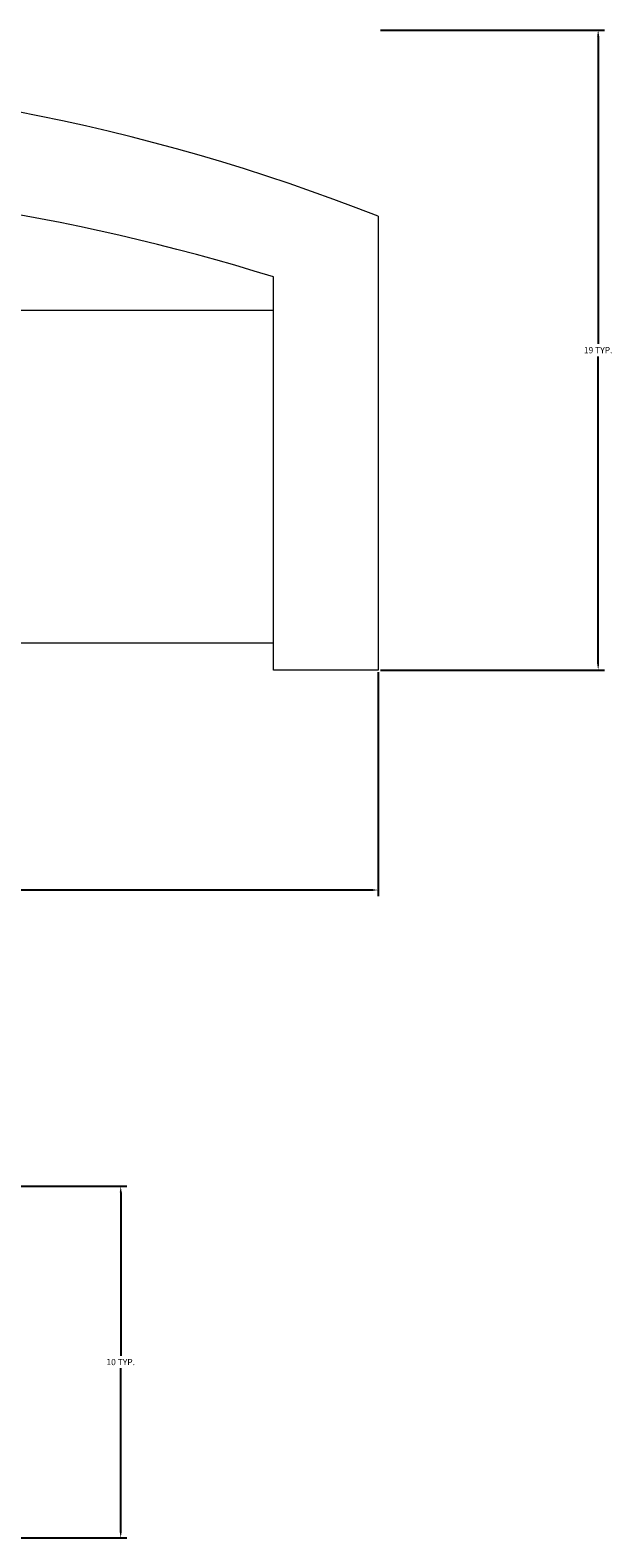
# Model space of a CAD drawing. Units: feet. Extents: x 2219 to 3039, y 1768 to 2369.
# Tile 10 of 16: x 2764 to 2781, y 2273 to 2317. Entities that reach past the tile are written whole.
import ezdxf

# ---------------------------------------------------------------- set-up
doc = ezdxf.new("R2010")
doc.units = ezdxf.units.FT
doc.layers.add('A-ANNO-DIMS', color=2, linetype='Continuous', lineweight=18)
doc.layers.add('A-FURN', color=8, linetype='Continuous', lineweight=18)
doc.styles.get("Standard").update_dxf_attribs({"font": 'arial.ttf'})
doc.dimstyles.get("Standard").update_dxf_attribs({"dimtxt": 0.18, "dimasz": 0.18, "dimexe": 0.18, "dimexo": 0.0625, "dimgap": 0.09, "dimtad": 0, "dimtih": 1, "dimtoh": 1, "dimdec": 4, "dimzin": 0, "dimdsep": 46, "dimtxsty": 'Standard', "dimcen": 0.09, "dimadec": 0, "dimazin": 0, "dimtfac": 1, "dimtdec": 4, "dimtofl": 0, "dimtmove": 0, "dimatfit": 3, "dimfxl": 1, "dimtolj": 1, "dimtzin": 0, "dimarcsym": 0})

# ---------------------------------------------------------------- blocks, each defined once
blk = doc.blocks.new('Sofa - Roundback 7 ft.')
for p, q in [((-12.00002, -32.4421), (-12.00003, -6.5971)), ((11.99997, -32.4421), (11.99998, -6.5971)), ((-36.000027, -34), (-36.000027, -11.4696)), ((35.99998, -34), (35.99998, -11.4696)), ((-35.999844, -13.3819), (35.9998, -13.3819)), ((-36.000027, -32.4421), (35.99998, -32.4421))]:
    blk.add_line(p, q)
for points in [[(-36.000027, -34), (-42.000027, -34), (-42.000027, -8)], [(41.99998, -8), (41.99998, -34), (35.99998, -34)]]:
    blk.add_lwpolyline(points)
for centre, radius, start, end in [((0, -114.25), 114.25, 68.43141, 111.5686), ((-0.00001, -127.1968), 121.1968, 72.72033, 107.2797)]:
    blk.add_arc(centre, radius, start, end)
blk = doc.blocks.new('*D24')
at = {"layer": 'A-ANNO-DIMS', "color": 0, "lineweight": -2, "transparency": 16777216}
for p, q in [((2731.366, 2298.238), (2731.366, 2291.74)), ((2773.903, 2298.238), (2773.903, 2291.74)), ((2731.546, 2291.92), (2751.73, 2291.92)), ((2773.723, 2291.92), (2753.54, 2291.92))]:
    blk.add_line(p, q, dxfattribs=at)
at = {"layer": 'A-ANNO-DIMS', "color": 0, "transparency": 16777216}
for points in [[(2731.546, 2291.95), (2731.546, 2291.89), (2731.366, 2291.92)], [(2773.723, 2291.95), (2773.723, 2291.89), (2773.903, 2291.92)]]:
    blk.add_solid(points, dxfattribs=at)
at = {"layer": 'Defpoints', "color": 0, "transparency": 16777216}
for p in [(2731.366, 2298.3), (2773.903, 2298.3), (2773.903, 2291.92)]:
    blk.add_point(p, dxfattribs=at)
at = {"layer": 'A-ANNO-DIMS', "color": 0, "transparency": 16777216, "insert": (2752.635, 2291.92), "char_height": 0.18, "attachment_point": 5}
blk.add_mtext('\\A1;SOFA 43 TYP.', dxfattribs=at)
blk = doc.blocks.new('*D25')
at = {"layer": 'A-ANNO-DIMS', "color": 0, "lineweight": -2, "transparency": 16777216}
for p, q in [((2773.966, 2316.868), (2780.464, 2316.868)), ((2780.284, 2316.688), (2780.284, 2307.766)), ((2780.284, 2298.48), (2780.284, 2307.402)), ((2773.966, 2298.3), (2780.464, 2298.3))]:
    blk.add_line(p, q, dxfattribs=at)
at = {"layer": 'A-ANNO-DIMS', "color": 0, "transparency": 16777216}
for points in [[(2780.254, 2316.688), (2780.314, 2316.688), (2780.284, 2316.868)], [(2780.254, 2298.48), (2780.314, 2298.48), (2780.284, 2298.3)]]:
    blk.add_solid(points, dxfattribs=at)
at = {"layer": 'Defpoints', "color": 0, "transparency": 16777216}
for p in [(2773.903, 2316.868), (2780.284, 2316.868), (2773.903, 2298.3)]:
    blk.add_point(p, dxfattribs=at)
at = {"layer": 'A-ANNO-DIMS', "color": 0, "transparency": 16777216, "insert": (2780.284, 2307.584), "char_height": 0.18, "attachment_point": 5}
blk.add_mtext('\\A1;19 TYP.', dxfattribs=at)
blk = doc.blocks.new('*D29')
at = {"layer": 'A-ANNO-DIMS', "color": 0, "lineweight": -2, "transparency": 16777216}
for p, q in [((2763.438, 2283.324), (2766.615, 2283.324)), ((2766.435, 2283.144), (2766.435, 2278.405)), ((2766.435, 2273.303), (2766.435, 2278.042)), ((2763.438, 2273.123), (2766.615, 2273.123))]:
    blk.add_line(p, q, dxfattribs=at)
at = {"layer": 'A-ANNO-DIMS', "color": 0, "transparency": 16777216}
for points in [[(2766.405, 2283.144), (2766.465, 2283.144), (2766.435, 2283.324)], [(2766.405, 2273.303), (2766.465, 2273.303), (2766.435, 2273.123)]]:
    blk.add_solid(points, dxfattribs=at)
at = {"layer": 'Defpoints', "color": 0, "transparency": 16777216}
for p in [(2763.375, 2283.324), (2766.435, 2283.324), (2763.375, 2273.123)]:
    blk.add_point(p, dxfattribs=at)
at = {"layer": 'A-ANNO-DIMS', "color": 0, "transparency": 16777216, "insert": (2766.435, 2278.224), "char_height": 0.18, "attachment_point": 5}
blk.add_mtext('\\A1;10 TYP.', dxfattribs=at)

msp = doc.modelspace()

# ---------------------------------------------------------------- block references
at = {"layer": 'A-FURN', "xscale": 0.5063942958922181, "yscale": 0.5063942958922181, "zscale": 0.5063942958922181}
msp.add_blockref('Sofa - Roundback 7 ft.', (2752.635, 2315.518), dxfattribs=at)

# ---------------------------------------------------------------- dimensions: what is measured, and where the dimension line sits
at = {"layer": 'A-ANNO-DIMS'}
for base, p1, p2, picture, middle in [((2780.284, 2316.868), (2773.903, 2298.3), (2773.903, 2316.868), '*D25', (2780.284, 2307.584)), ((2766.435, 2283.324), (2763.375, 2273.123), (2763.375, 2283.324), '*D29', (2766.435, 2278.224))]:
    dim = msp.add_linear_dim(base=base, p1=p1, p2=p2, angle=90, text='<> TYP.', dimstyle='Standard', override={"dimdec": 0, "dimlfac": 1, "dimrnd": 0, "dimzin": 0, "dimdsep": 46, "dimlunit": 2}, dxfattribs=at)
    dim.commit()
    dim.dimension.update_dxf_attribs({"geometry": picture, "text_midpoint": middle})
dim = msp.add_linear_dim(base=(2773.903, 2291.92), p1=(2731.366, 2298.3), p2=(2773.903, 2298.3), text='SOFA <> TYP.', dimstyle='Standard', override={"dimdec": 0, "dimlfac": 1, "dimrnd": 0, "dimzin": 0, "dimdsep": 46, "dimlunit": 2}, dxfattribs=at)
dim.commit()
dim.dimension.update_dxf_attribs({"geometry": '*D24', "text_midpoint": (2752.635, 2291.92)})

doc.saveas('drawing.dxf')
